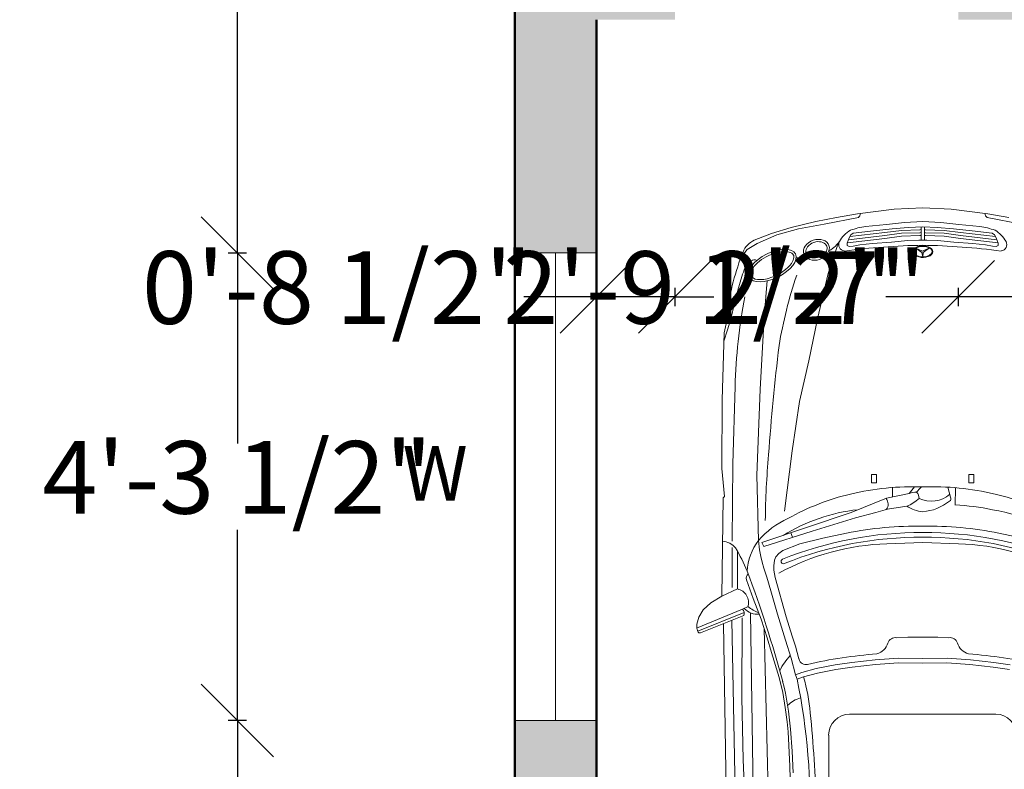
# Model space of a CAD drawing. Units: inches. Extents: x 3121 to 3511, y 1323 to 1998.
# Tile 3 of 10: x 3135 to 3244, y 1456 to 1539. Entities that reach past the tile are written whole.
import ezdxf

# ---------------------------------------------------------------- set-up
doc = ezdxf.new("R2010")
doc.units = ezdxf.units.IN
for name, color, linetype, lineweight in [('0_Equip', 250, 'Continuous', 13), ('A-ANNO-DIMS', 2, 'Continuous', 18), ('A-ANNO-TEXT', 7, 'Continuous', 18), ('A-GLAZ', 4, 'Continuous', 18), ('A-WALL', 7, 'Continuous', 50), ('A-WALL-PATT', 3, 'Continuous', 13)]:
    doc.layers.add(name, color=color, linetype=linetype, lineweight=lineweight)
doc.styles.get("Standard").update_dxf_attribs({"font": 'arial.ttf'})
doc.dimstyles.new('ISO-25', dxfattribs={"dimtxt": 8, "dimasz": 8, "dimexe": 1, "dimexo": 1, "dimtad": 0, "dimtih": 1, "dimtoh": 1, "dimlunit": 3, "dimtxsty": 'Standard', "dimblk": 'OBLIQUE', "dimcen": 2.5, "dimclrt": 1, "dimadec": 0, "dimazin": 0, "dimtfac": 1, "dimtmove": 0, "dimatfit": 3, "dimfxl": 1, "dimfxlon": 1, "dimarcsym": 0})

# ---------------------------------------------------------------- blocks, each defined once
blk = doc.blocks.new('A$C4C7B54D1')
at = {"layer": '0_Equip', "ltscale": 0.1}
for p, q in [((-1.0176, 2.6505), (-1.112, 2.6343)), ((-0.8531, 2.6707), (-1.0176, 2.6505)), ((-0.7257, 2.678), (-0.8531, 2.6707)), ((-0.7257, 2.678), (-0.5983, 2.6707)), ((-0.5983, 2.6707), (-0.4338, 2.6505)), ((-0.4338, 2.6505), (-0.3394, 2.6343)), ((-1.2037, 2.6168), (-1.3142, 2.5898)), ((-1.1673, 2.6045), (-1.2824, 2.5829)), ((-1.112, 2.6343), (-1.2037, 2.6168)), ((-1.0138, 2.6343), (-1.1673, 2.6045)), ((-0.8877, 2.6027), (-0.9812, 2.5937)), ((-0.8072, 2.6112), (-0.8877, 2.6027)), ((-0.7257, 2.6157), (-0.8072, 2.6112)), ((-0.7257, 2.6157), (-0.6441, 2.6112)), ((-0.6441, 2.6112), (-0.5636, 2.6027)), ((-0.5636, 2.6027), (-0.4701, 2.5937)), ((-0.4376, 2.6343), (-0.284, 2.6045)), ((-1.4032, 2.5628), (-1.4801, 2.5318)), ((-1.3142, 2.5898), (-1.4032, 2.5628)), ((-1.2824, 2.5829), (-1.3789, 2.557)), ((-1.4667, 2.5181), (-1.5113, 2.4907)), ((-1.3789, 2.557), (-1.4667, 2.5181)), ((-1.5113, 2.4907), (-1.5393, 2.4562)), ((-1.1083, 2.5037), (-1.1486, 2.3827)), ((-1.1486, 2.3827), (-1.1961, 2.1797)), ((-1.5353, 2.3701), (-1.5529, 2.308)), ((-1.435, 2.1869), (-1.4221, 2.3511)), ((-1.5529, 2.308), (-1.5677, 2.2486)), ((-1.5677, 2.2486), (-1.5849, 2.1795)), ((-1.6012, 2.2082), (-1.597, 2.1976)), ((-1.597, 2.1976), (-1.615, 2.1169)), ((-1.5849, 2.1795), (-1.5997, 2.1304)), ((-1.4537, 1.863), (-1.435, 2.1869)), ((-1.1961, 2.1797), (-1.2349, 1.9911)), ((-1.615, 2.1169), (-1.6235, 1.8165)), ((-1.5997, 2.1304), (-1.6161, 2.0798)), ((-1.2349, 1.9911), (-1.2767, 1.8097)), ((-1.566, 1.8774), (-1.5761, 1.5304)), ((-1.4681, 1.48), (-1.4537, 1.863)), ((-1.6235, 1.8165), (-1.6256, 1.5098)), ((-1.2767, 1.8097), (-1.3098, 1.588)), ((-1.3098, 1.588), (-1.3443, 1.3187)), ((-1.6256, 1.5098), (-1.6129, 1.3846)), ((-1.5761, 1.5304), (-1.5789, 1.1834)), ((-1.461, 1.1868), (-1.4681, 1.48)), ((-0.955, 1.4459), (-0.955, 1.4827)), ((-0.955, 1.4827), (-0.9321, 1.4827)), ((-0.9321, 1.4827), (-0.9321, 1.4459)), ((-0.5192, 1.4827), (-0.5192, 1.4459)), ((-0.4964, 1.4827), (-0.5192, 1.4827)), ((-0.4964, 1.4459), (-0.4964, 1.4827)), ((-0.9321, 1.4459), (-0.955, 1.4459)), ((-0.8614, 1.4242), (-0.8603, 1.382)), ((-0.6135, 1.4258), (-0.6012, 1.3814)), ((-0.5809, 1.3459), (-0.5793, 1.4233)), ((-0.5192, 1.4459), (-0.4964, 1.4459)), ((-1.6193, 1.3782), (-1.6252, 0.9375)), ((-1.6129, 1.3846), (-1.6193, 1.3782)), ((-0.8878, 1.3764), (-1.0456, 1.313)), ((-0.7861, 1.3973), (-0.8878, 1.3764)), ((-0.9361, 1.3119), (-0.8835, 1.3269)), ((-0.8835, 1.3269), (-0.7975, 1.3408)), ((-1.0456, 1.313), (-1.4462, 1.1776)), ((-1.2207, 1.2292), (-1.0263, 1.2883)), ((-1.0263, 1.2883), (-0.9361, 1.3119)), ((-1.4366, 1.1604), (-1.2207, 1.2292)), ((-1.3162, 1.2215), (-1.3088, 1.2011)), ((-1.1723, 1.1976), (-1.2762, 1.1716)), ((-1.0667, 1.22), (-1.1723, 1.1976)), ((-0.3847, 1.22), (-0.279, 1.1976)), ((-1.5793, 1.1562), (-1.5793, 0.9761)), ((-1.4565, 1.1447), (-1.461, 1.1868)), ((-1.4462, 1.1776), (-1.4366, 1.1604)), ((-1.2762, 1.1716), (-1.3515, 1.142)), ((-0.7257, 1.1776), (-0.8858, 1.1725)), ((-0.7257, 1.1776), (-0.5655, 1.1725)), ((-1.5552, 1.139), (-1.5552, 0.9693)), ((-1.4503, 1.1151), (-1.4565, 1.1447)), ((-1.444, 1.0892), (-1.4503, 1.1151)), ((-1.3828, 1.1133), (-1.39, 1.0981)), ((-1.3703, 1.1286), (-1.3828, 1.1133)), ((-1.3515, 1.142), (-1.3703, 1.1286)), ((-1.4368, 1.0623), (-1.444, 1.0892)), ((-1.4243, 1.0229), (-1.4368, 1.0623)), ((-1.39, 1.0981), (-1.3927, 1.0739)), ((-1.3927, 1.0739), (-1.3918, 1.0533)), ((-1.4064, 0.961), (-1.4243, 1.0229)), ((-1.3918, 1.0533), (-1.3867, 1.0211)), ((-1.3867, 1.0211), (-1.3374, 0.8446)), ((-1.5149, 1.011), (-1.4844, 0.9277)), ((-1.6252, 0.9375), (-1.6745, 0.908)), ((-1.6252, 0.9375), (-1.5546, 0.9696)), ((-1.4844, 0.9277), (-1.4486, 0.8345)), ((-1.3759, 0.8562), (-1.4064, 0.961)), ((-1.6745, 0.908), (-1.7088, 0.8764)), ((-1.508, 0.8914), (-1.5321, 0.8786)), ((-1.5321, 0.8786), (-1.7381, 0.7945)), ((-1.728, 0.8432), (-1.7366, 0.8127)), ((-1.5253, 0.865), (-1.7329, 0.7802)), ((-1.7088, 0.8764), (-1.728, 0.8432)), ((-1.5273, 0.8512), (-1.7203, 0.7738)), ((-1.5337, 0.8406), (-1.5355, 0.484)), ((-1.4835, -0.0735), (-1.497, 0.863)), ((-1.3401, 0.7406), (-1.3759, 0.8562)), ((-1.3374, 0.8446), (-1.3097, 0.7577)), ((-1.7366, 0.8127), (-1.7377, 0.7934)), ((-1.6171, 0.8152), (-1.5964, -0.6171)), ((-1.5805, 0.8299), (-1.5623, -0.138)), ((-1.4486, 0.8345), (-1.4226, 0.7503)), ((-1.7377, 0.7934), (-1.7327, 0.7794)), ((-1.4352, 0.792), (-1.4152, -0.045)), ((-1.4226, 0.7503), (-1.4029, 0.6849)), ((-1.3097, 0.7577), (-1.2953, 0.7129)), ((-0.7926, 0.7532), (-0.8418, 0.7514)), ((-0.7257, 0.7541), (-0.7926, 0.7532)), ((-0.7257, 0.7541), (-0.6587, 0.7532)), ((-0.6587, 0.7532), (-0.6095, 0.7514)), ((-1.315, 0.66), (-1.3401, 0.7406)), ((-1.2953, 0.7129), (-1.2801, 0.6573)), ((-1.4029, 0.6849), (-1.368, 0.5729)), ((-1.2951, 0.5849), (-1.315, 0.66)), ((-1.2801, 0.6573), (-1.2795, 0.6546)), ((-1.1177, 0.6302), (-1.2021, 0.6133)), ((-1.0437, 0.6403), (-1.1177, 0.6302)), ((-1.0411, 0.6196), (-1.1142, 0.6096)), ((-0.9389, 0.6526), (-1.0437, 0.6403)), ((-0.937, 0.6317), (-1.0411, 0.6196)), ((-0.8346, 0.6593), (-0.9389, 0.6526)), ((-0.834, 0.6384), (-0.937, 0.6317)), ((-0.7257, 0.6582), (-0.8346, 0.6593)), ((-0.7257, 0.6373), (-0.834, 0.6384)), ((-0.7257, 0.6582), (-0.6168, 0.6593)), ((-0.7257, 0.6373), (-0.6173, 0.6384)), ((-0.6173, 0.6384), (-0.5143, 0.6317)), ((-0.6168, 0.6593), (-0.5124, 0.6526)), ((-0.5143, 0.6317), (-0.4102, 0.6196)), ((-0.5124, 0.6526), (-0.4076, 0.6403)), ((-0.4102, 0.6196), (-0.3371, 0.6096)), ((-0.4076, 0.6403), (-0.3337, 0.6302)), ((-1.2663, 0.5956), (-1.2951, 0.5849)), ((-1.2879, 0.5653), (-1.2951, 0.5849)), ((-1.2599, 0.5757), (-1.2879, 0.5653)), ((-1.2021, 0.6133), (-1.2663, 0.5956)), ((-1.1973, 0.593), (-1.2599, 0.5757)), ((-1.1142, 0.6096), (-1.1973, 0.593)), ((-1.368, 0.5729), (-1.3527, 0.5066)), ((-1.3527, 0.5066), (-1.3411, 0.4394)), ((-1.5355, 0.484), (-1.5292, 0.2045)), ((-1.3411, 0.4394), (-1.3321, 0.3749)), ((-0.7257, 0.4085), (-1.0528, 0.4085)), ((-0.7257, 0.4085), (-0.3986, 0.4085)), ((-1.3321, 0.3749), (-1.3286, 0.3301)), ((-1.3286, 0.3301), (-1.3204, 0.1751)), ((-1.3178, 0.3418), (-1.31, 0.2426)), ((-1.1468, 0.3145), (-1.1468, 0.0145)), ((-1.31, 0.2426), (-1.306, 0.1454)), ((-1.5292, 0.2045), (-1.5185, -0.0974)), ((-1.3204, 0.1751), (-1.3164, 0.0193))]:
    blk.add_line(p, q, dxfattribs=at)
at = {"layer": '0_Equip'}
for p, q in [((-1.0475, 2.557), (-1.0545, 2.5425)), ((-1.0517, 2.5482), (-0.8949, 2.567)), ((-1.0364, 2.5634), (-1.0475, 2.557)), ((-0.9467, 2.5739), (-1.0364, 2.5634)), ((-0.8628, 2.5838), (-0.9467, 2.5739)), ((-0.8949, 2.567), (-0.8211, 2.5763)), ((-0.8949, 2.5537), (-0.8211, 2.5631)), ((-0.7905, 2.5897), (-0.8628, 2.5838)), ((-0.8211, 2.5763), (-0.738, 2.5791)), ((-0.8211, 2.5631), (-0.738, 2.5659)), ((-0.7257, 2.5926), (-0.7905, 2.5897)), ((-0.738, 2.5791), (-0.733, 2.58)), ((-0.738, 2.5659), (-0.733, 2.5668)), ((-0.733, 2.5923), (-0.733, 2.5325)), ((-0.7257, 2.5926), (-0.6608, 2.5897)), ((-0.7183, 2.5923), (-0.7183, 2.5325)), ((-0.7133, 2.5791), (-0.7183, 2.58)), ((-0.7133, 2.5659), (-0.7183, 2.5668)), ((-0.6302, 2.5763), (-0.7133, 2.5791)), ((-0.6302, 2.5631), (-0.7133, 2.5659)), ((-0.6608, 2.5897), (-0.5886, 2.5838)), ((-0.5564, 2.567), (-0.6302, 2.5763)), ((-0.5564, 2.5537), (-0.6302, 2.5631)), ((-0.5886, 2.5838), (-0.5046, 2.5739)), ((-0.3996, 2.5482), (-0.5564, 2.567)), ((-0.5046, 2.5739), (-0.4149, 2.5634)), ((-0.4149, 2.5634), (-0.4038, 2.557)), ((-0.4038, 2.557), (-0.3968, 2.5425)), ((-1.0545, 2.5425), (-1.0638, 2.5185)), ((-1.0638, 2.5185), (-1.0638, 2.5092)), ((-1.0631, 2.5204), (-0.8949, 2.5405)), ((-1.0577, 2.5343), (-0.8949, 2.5537)), ((-1.0067, 2.5116), (-0.9502, 2.5168)), ((-0.9502, 2.5168), (-0.8657, 2.5238)), ((-0.8949, 2.5405), (-0.8211, 2.5498)), ((-0.8657, 2.5238), (-0.7922, 2.5308)), ((-0.8211, 2.5498), (-0.738, 2.5526)), ((-0.7922, 2.5308), (-0.7433, 2.5325)), ((-0.7433, 2.5325), (-0.7257, 2.5325)), ((-0.738, 2.5526), (-0.733, 2.5536)), ((-0.708, 2.5325), (-0.7257, 2.5325)), ((-0.7133, 2.5526), (-0.7183, 2.5536)), ((-0.6302, 2.5498), (-0.7133, 2.5526)), ((-0.6591, 2.5308), (-0.708, 2.5325)), ((-0.5857, 2.5238), (-0.6591, 2.5308)), ((-0.5564, 2.5405), (-0.6302, 2.5498)), ((-0.5011, 2.5168), (-0.5857, 2.5238)), ((-0.3936, 2.5343), (-0.5564, 2.5537)), ((-0.3882, 2.5204), (-0.5564, 2.5405)), ((-0.4446, 2.5116), (-0.5011, 2.5168)), ((-0.3968, 2.5425), (-0.3875, 2.5185)), ((-0.3875, 2.5185), (-0.3875, 2.5092)), ((-1.0638, 2.5092), (-1.0545, 2.504)), ((-1.0545, 2.504), (-1.0376, 2.5051)), ((-1.0376, 2.5051), (-1.0067, 2.5116)), ((-0.7566, 2.4971), (-0.7261, 2.4828)), ((-0.7566, 2.4971), (-0.7291, 2.4776)), ((-0.7389, 2.5095), (-0.7395, 2.5059)), ((-0.7259, 2.4578), (-0.7291, 2.4776)), ((-0.6947, 2.4974), (-0.7261, 2.4828)), ((-0.7259, 2.4578), (-0.723, 2.4776)), ((-0.6947, 2.4974), (-0.723, 2.4776)), ((-0.7124, 2.5095), (-0.7119, 2.5059)), ((-0.4137, 2.5051), (-0.4446, 2.5116)), ((-0.3968, 2.504), (-0.4137, 2.5051)), ((-0.3875, 2.5092), (-0.3968, 2.504))]:
    blk.add_line(p, q, dxfattribs=at)
at = {"layer": '0_Equip', "ltscale": 0.1}
for centre, radius, start, end in [((-1.0252, 2.6508), 0.02, 304.7228, 3.5172), ((-0.4261, 2.6508), 0.02, 176.4828, 235.2772), ((-0.9799, 2.461), 0.1353, 120.8369, 151.2853), ((-0.9299, 2.2354), 0.3619, 98.1466, 109.2524), ((-0.5214, 2.2354), 0.3619, 70.7476, 81.8534), ((-0.4714, 2.461), 0.1353, 28.7147, 59.1631), ((-1.4391, 2.4422), 0.0986, 114.5945, 157.5113), ((-1.2153, 2.6098), 0.1432, 299.1564, 328.1831), ((-0.9799, 2.461), 0.1353, 151.2853, 161.5889), ((-1.0728, 2.5126), 0.029, 152.6038, 261.721), ((-0.3785, 2.5126), 0.029, 278.279, 27.3962), ((-0.4722, 2.0579), 1.139, 158.2564, 172.4203), ((-0.6679, -0.6671), 3.1773, 91.0415, 97.3969), ((-0.7834, -0.6671), 3.1773, 82.6031, 88.9585), ((-1.4083, 2.3394), 0.1306, 130.2084, 166.4224), ((-1.4798, 2.4259), 0.0184, 54.8052, 134.0204), ((-1.2841, 2.5028), 0.0501, 260.5448, 306.7068), ((0.5502, 1.746), 1.9445, 161.1117, 170.7019), ((1.1202, 1.7918), 2.6875, 169.5541, 178.1755), ((9.2655, 0.7813), 10.7109, 173.14258, 175.77374), ((2.9623, 1.2089), 4.3935, 175.2767, 179.1124), ((-0.7686, 0.201), 1.2267, 87.9955, 103.2364), ((-0.3726, 1.0935), 0.5131, 139.3585, 143.6922), ((-0.6528, 1.3354), 0.1211, 130.7679, 145.6911), ((-0.6828, 0.201), 1.2267, 76.7636, 92.0045), ((-0.786, 0.3109), 1.1158, 103.6551, 119.1148), ((-0.9216, 1.3498), 0.0409, 323.4512, 39.0343), ((-0.8494, 1.486), 0.1542, 289.6676, 314.192), ((-0.7554, 1.327), 0.0768, 88.1186, 113.6019), ((-0.7803, 1.3768), 0.0384, 357.9275, 44.3829), ((-0.6872, 1.4869), 0.1241, 243.8649, 311.6638), ((-0.6113, 1.3746), 0.0122, 294.8678, 33.6398), ((-0.6653, 0.3109), 1.1158, 60.8852, 76.3449), ((-0.929, 0.5266), 0.803, 96.22, 121.6991), ((-0.7147, 1.4628), 0.1474, 235.8143, 265.7174), ((-0.741, 1.5272), 0.212, 274.1513, 309.4931), ((-0.617, 0.3882), 0.9584, 77.6919, 87.8428), ((-0.5976, 0.2949), 1.0461, 55.3038, 79.8165), ((-1.1803, 0.9494), 0.3676, 113.8511, 139.7847), ((-0.7478, -0.378), 1.6295, 89.2231, 101.2856), ((-0.7036, -0.378), 1.6295, 78.7144, 90.7769), ((-0.7356, -0.4312), 1.6538, 89.6554, 111.9286), ((-0.7356, -0.4312), 1.6329, 89.6554, 111.9286), ((-0.7157, -0.4312), 1.6538, 68.0714, 90.3446), ((-0.7157, -0.4312), 1.6329, 68.0714, 90.3446), ((-1.6261, 1.102), 0.0813, 40.278, 87.0689), ((-2.3477, 0.6968), 0.9076, 22.824, 30.2904), ((-1.2706, 1.0395), 0.2408, 142.2718, 177.7746), ((-0.85, 0.0855), 1.0875, 91.8892, 118.6013), ((-0.6014, 0.0855), 1.0875, 61.3987, 88.1108), ((-1.3493, 1.0932), 0.0105, 111.9286, 291.9286), ((-1.4887, 1.0171), 0.0269, 132.3277, 193.1064), ((-6.6059, -0.8606), 5.4408, 15.0904, 20.5451), ((-1.5684, 0.9084), 0.0628, 344.3283, 77.2348), ((-1.463, 0.9441), 0.0879, 224.7932, 273.9292), ((-1.4233, 0.9849), 0.1262, 227.8287, 253.081), ((-1.5495, 0.8614), 0.0245, 335.4987, 44.5114), ((-1.7238, 0.7825), 0.00941, 199.646, 291.8616), ((-0.8474, 0.7163), 0.0355, 80.937, 162.15), ((-0.6039, 0.7163), 0.0355, 17.85, 99.063), ((-0.9515, 0.7495), 0.0737, 286.567, 342.4011), ((-0.4998, 0.7495), 0.0737, 197.5989, 253.433), ((-1.1535, 0.5061), 0.2334, 134.9877, 155.4049), ((-0.7896, -1.2957), 1.9795, 94.0807, 103.2045), ((-0.6617, -1.2957), 1.9795, 76.7955, 85.9193), ((-1.249, 0.662), 0.0314, 193.667, 283.2045), ((-2.0025, 0.3511), 0.7759, 4.7259, 16.8296), ((-2.6334, 0.2371), 1.3197, 4.5498, 13.9797), ((-4.2099, -0.0242), 2.9809, 358.1905, 11.4064), ((-1.2324, 0.3484), 0.1397, 106.6168, 134.6647), ((-6.5594, -0.126), 5.3575, 1.3159, 5.7952), ((-1.0528, 0.3145), 0.0941, 90, 180), ((-0.3986, 0.3145), 0.0941, 0, 90)]:
    blk.add_arc(centre, radius, start, end, dxfattribs=at)
for centre, major_axis, ratio in [((-1.2016, 2.4892), (0.0562, 0.0189), 0.759763), ((-1.399, 2.4187), (-0.1036, -0.0518), 0.497493)]:
    blk.add_ellipse(centre, major_axis=major_axis, ratio=ratio, dxfattribs=at)
at = {"layer": '0_Equip'}
blk.add_ellipse((-0.7253, 2.4812), major_axis=(-0.0426, 0), ratio=0.550187, dxfattribs=at)
at = {"layer": '0_Equip', "ltscale": 0.1}
for points, knots in [([(-1.1548, 2.5048), (-1.1596, 2.5191), (-1.1811, 2.5294), (-1.2283, 2.5198), (-1.248, 2.5001), (-1.2511, 2.4679), (-1.2373, 2.4539), (-1.1922, 2.4512), (-1.1656, 2.4658), (-1.1532, 2.4906), (-1.1526, 2.4983), (-1.1548, 2.5048)], [0, 0, 0, 0, 1.408119, 1.408119, 2.816238, 2.816238, 4.224358, 4.224358, 5.632477, 5.632477, 6.283185, 6.283185, 6.283185, 6.283185]), ([(-1.4937, 2.3714), (-1.4901, 2.3641), (-1.4809, 2.3581), (-1.4492, 2.3543), (-1.4277, 2.3571), (-1.3679, 2.3771), (-1.3298, 2.404), (-1.2994, 2.4483), (-1.2993, 2.4626), (-1.3171, 2.4801), (-1.3406, 2.4849), (-1.3989, 2.4733), (-1.4323, 2.4577), (-1.4816, 2.4186), (-1.4956, 2.3954), (-1.4959, 2.3774), (-1.4951, 2.3742), (-1.4937, 2.3714)], [0, 0, 0, 0, 0.646556, 0.646556, 1.293113, 1.293113, 2.410172, 2.410172, 3.309931, 3.309931, 4.20969, 4.20969, 5.109449, 5.109449, 6.031285, 6.031285, 6.283185, 6.283185, 6.283185, 6.283185])]:
    blk.add_open_spline(points, degree=3, knots=knots, dxfattribs=at)
at = {"layer": '0_Equip'}
blk.add_open_spline([(-0.7708, 2.4812), (-0.7708, 2.4725), (-0.7635, 2.4648), (-0.7294, 2.4499), (-0.6897, 2.4563), (-0.6733, 2.4916), (-0.7036, 2.5102), (-0.7526, 2.5051), (-0.7708, 2.4948), (-0.7708, 2.4812)], degree=3, knots=[0, 0, 0, 0, 0.903923, 0.903923, 2.878844, 2.878844, 4.872977, 4.872977, 6.283185, 6.283185, 6.283185, 6.283185], dxfattribs=at)
blk = doc.blocks.new('_Oblique')
at = {"color": 0, "linetype": 'ByBlock', "lineweight": -2}
blk.add_line((-0.5, -0.5), (0.5, 0.5), dxfattribs=at)
blk = doc.blocks.new('*D35')
at = {"layer": 'A-ANNO-DIMS', "color": 0, "lineweight": -2, "transparency": 16777216}
for p, q in [((3160.37, 1461.55), (3158.37, 1461.55)), ((3159.37, 1461.55), (3159.37, 1443.38)), ((3159.37, 1415.78), (3159.37, 1433.95)), ((3160.37, 1415.78), (3158.37, 1415.78))]:
    blk.add_line(p, q, dxfattribs=at)
at = {"layer": 'Defpoints', "color": 0, "transparency": 16777216}
for p in [(3159.37, 1461.55), (3189.92, 1461.55), (3189.92, 1415.78)]:
    blk.add_point(p, dxfattribs=at)
at = {"layer": 'A-ANNO-DIMS', "color": 0, "lineweight": -2, "transparency": 16777216, "xscale": 8, "yscale": 8, "zscale": 8}
for p, rotation in [((3159.37, 1461.55), 90), ((3159.37, 1415.78), 270)]:
    blk.add_blockref('_Oblique', p, dxfattribs=dict(at, rotation=rotation))
at = {"layer": 'A-ANNO-DIMS', "color": 1, "transparency": 16777216, "insert": (3159.37, 1438.67), "char_height": 8, "attachment_point": 5}
blk.add_mtext('3\'-10"', dxfattribs=at)
blk = doc.blocks.new('*D36')
at = {"layer": 'A-ANNO-DIMS', "color": 0, "lineweight": -2, "transparency": 16777216}
for p, q in [((3160.37, 1513.07), (3158.37, 1513.07)), ((3159.37, 1513.07), (3159.37, 1492.07)), ((3159.37, 1461.55), (3159.37, 1482.55)), ((3160.37, 1461.55), (3158.37, 1461.55))]:
    blk.add_line(p, q, dxfattribs=at)
at = {"layer": 'Defpoints', "color": 0, "transparency": 16777216}
for p in [(3159.37, 1513.07), (3189.92, 1513.07), (3189.92, 1461.55)]:
    blk.add_point(p, dxfattribs=at)
at = {"layer": 'A-ANNO-DIMS', "color": 0, "lineweight": -2, "transparency": 16777216, "xscale": 8, "yscale": 8, "zscale": 8}
for p, rotation in [((3159.37, 1513.07), 90), ((3159.37, 1461.55), 270)]:
    blk.add_blockref('_Oblique', p, dxfattribs=dict(at, rotation=rotation))
at = {"layer": 'A-ANNO-DIMS', "color": 1, "transparency": 16777216, "insert": (3159.37, 1487.31), "char_height": 8, "attachment_point": 5}
blk.add_mtext('4\'-3 1/2"', dxfattribs=at)
blk = doc.blocks.new('*D37')
at = {"layer": 'A-ANNO-DIMS', "color": 0, "lineweight": -2, "transparency": 16777216}
for p, q in [((3160.37, 1607.33), (3158.37, 1607.33)), ((3159.37, 1607.33), (3159.37, 1564.96)), ((3159.37, 1513.07), (3159.37, 1555.44)), ((3160.37, 1513.07), (3158.37, 1513.07))]:
    blk.add_line(p, q, dxfattribs=at)
at = {"layer": 'Defpoints', "color": 0, "transparency": 16777216}
for p in [(3159.37, 1607.33), (3189.92, 1607.33), (3189.92, 1513.07)]:
    blk.add_point(p, dxfattribs=at)
at = {"layer": 'A-ANNO-DIMS', "color": 0, "lineweight": -2, "transparency": 16777216, "xscale": 8, "yscale": 8, "zscale": 8}
for p, rotation in [((3159.37, 1607.33), 90), ((3159.37, 1513.07), 270)]:
    blk.add_blockref('_Oblique', p, dxfattribs=dict(at, rotation=rotation))
at = {"layer": 'A-ANNO-DIMS', "color": 1, "transparency": 16777216, "insert": (3159.37, 1560.2), "char_height": 8, "attachment_point": 5}
blk.add_mtext('7\'-10 1/2"', dxfattribs=at)
blk = doc.blocks.new('*D58')
at = {"layer": 'A-ANNO-DIMS', "color": 0, "lineweight": -2, "transparency": 16777216}
for p, q in [((3209.89, 1985.33), (3209.89, 1987.33)), ((3311.33, 1985.33), (3311.33, 1987.33)), ((3209.89, 1986.33), (3240.03, 1986.33)), ((3311.33, 1986.33), (3281.19, 1986.33))]:
    blk.add_line(p, q, dxfattribs=at)
at = {"layer": 'Defpoints', "color": 0, "transparency": 16777216}
for p in [(3311.33, 1986.33), (3209.89, 1424.78), (3311.33, 1424.78)]:
    blk.add_point(p, dxfattribs=at)
at = {"layer": 'A-ANNO-DIMS', "color": 0, "lineweight": -2, "transparency": 16777216, "xscale": 8, "yscale": 8, "zscale": 8, "rotation": 180}
blk.add_blockref('_Oblique', (3209.89, 1986.33), dxfattribs=at)
at = {"layer": 'A-ANNO-DIMS', "color": 0, "lineweight": -2, "transparency": 16777216, "xscale": 8, "yscale": 8, "zscale": 8}
blk.add_blockref('_Oblique', (3311.33, 1986.33), dxfattribs=at)
at = {"layer": 'A-ANNO-DIMS', "color": 1, "transparency": 16777216, "insert": (3260.61, 1986.33), "char_height": 8, "attachment_point": 5}
blk.add_mtext('8\'-5 1/2"', dxfattribs=at)
blk = doc.blocks.new('*D67')
at = {"layer": 'A-ANNO-DIMS', "color": 0, "lineweight": -2, "transparency": 16777216}
for p, q in [((3198.92, 1509.23), (3198.92, 1507.23)), ((3207.56, 1509.23), (3207.56, 1507.23)), ((3198.92, 1508.23), (3190.92, 1508.23)), ((3207.56, 1508.23), (3198.92, 1508.23))]:
    blk.add_line(p, q, dxfattribs=at)
at = {"layer": 'Defpoints', "color": 0, "transparency": 16777216}
for p in [(3198.92, 1538.78), (3207.56, 1538.78), (3198.92, 1508.23)]:
    blk.add_point(p, dxfattribs=at)
at = {"layer": 'A-ANNO-DIMS', "color": 0, "lineweight": -2, "transparency": 16777216, "xscale": 8, "yscale": 8, "zscale": 8, "rotation": 180}
blk.add_blockref('_Oblique', (3198.92, 1508.23), dxfattribs=at)
at = {"layer": 'A-ANNO-DIMS', "color": 0, "lineweight": -2, "transparency": 16777216, "xscale": 8, "yscale": 8, "zscale": 8}
blk.add_blockref('_Oblique', (3207.56, 1508.23), dxfattribs=at)
at = {"layer": 'A-ANNO-DIMS', "color": 1, "transparency": 16777216, "insert": (3170.34, 1508.23), "char_height": 8, "attachment_point": 5}
blk.add_mtext('0\'-8 1/2"', dxfattribs=at)
blk = doc.blocks.new('*D68')
at = {"layer": 'A-ANNO-DIMS', "color": 0, "lineweight": -2, "transparency": 16777216}
for p, q in [((3207.56, 1509.23), (3207.56, 1507.23)), ((3238.77, 1509.23), (3238.77, 1507.23)), ((3207.56, 1508.23), (3211.84, 1508.23)), ((3238.77, 1508.23), (3234.49, 1508.23))]:
    blk.add_line(p, q, dxfattribs=at)
at = {"layer": 'Defpoints', "color": 0, "transparency": 16777216}
for p in [(3207.56, 1538.78), (3238.77, 1538.78), (3207.56, 1508.23)]:
    blk.add_point(p, dxfattribs=at)
at = {"layer": 'A-ANNO-DIMS', "color": 0, "lineweight": -2, "transparency": 16777216, "xscale": 8, "yscale": 8, "zscale": 8, "rotation": 180}
blk.add_blockref('_Oblique', (3207.56, 1508.23), dxfattribs=at)
at = {"layer": 'A-ANNO-DIMS', "color": 0, "lineweight": -2, "transparency": 16777216, "xscale": 8, "yscale": 8, "zscale": 8}
blk.add_blockref('_Oblique', (3238.77, 1508.23), dxfattribs=at)
at = {"layer": 'A-ANNO-DIMS', "color": 1, "transparency": 16777216, "insert": (3223.16, 1508.23), "char_height": 8, "attachment_point": 5}
blk.add_mtext('2\'-7"', dxfattribs=at)
blk = doc.blocks.new('*D69')
at = {"layer": 'A-ANNO-DIMS', "color": 0, "lineweight": -2, "transparency": 16777216}
for p, q in [((3238.77, 1509.23), (3238.77, 1507.23)), ((3272.21, 1509.23), (3272.21, 1507.23)), ((3238.77, 1508.23), (3230.77, 1508.23)), ((3272.21, 1508.23), (3238.77, 1508.23))]:
    blk.add_line(p, q, dxfattribs=at)
at = {"layer": 'Defpoints', "color": 0, "transparency": 16777216}
for p in [(3238.77, 1538.78), (3272.21, 1538.78), (3238.77, 1508.23)]:
    blk.add_point(p, dxfattribs=at)
at = {"layer": 'A-ANNO-DIMS', "color": 0, "lineweight": -2, "transparency": 16777216, "xscale": 8, "yscale": 8, "zscale": 8, "rotation": 180}
blk.add_blockref('_Oblique', (3238.77, 1508.23), dxfattribs=at)
at = {"layer": 'A-ANNO-DIMS', "color": 0, "lineweight": -2, "transparency": 16777216, "xscale": 8, "yscale": 8, "zscale": 8}
blk.add_blockref('_Oblique', (3272.21, 1508.23), dxfattribs=at)
at = {"layer": 'A-ANNO-DIMS', "color": 1, "transparency": 16777216, "insert": (3210.12, 1508.23), "char_height": 8, "attachment_point": 5}
blk.add_mtext('2\'-9 1/2"', dxfattribs=at)

msp = doc.modelspace()

# ---------------------------------------------------------------- hatches: boundary and pattern name
at = {"layer": 'A-WALL-PATT'}
h = msp.add_hatch(color=256, dxfattribs=at)
h.dxf.hatch_style = 1
h.paths.add_polyline_path([(3274.023, 1955.784), (3189.918, 1955.784), (3189.918, 1910.219), (3198.918, 1910.219), (3198.918, 1946.784), (3259.023, 1946.784), (3259.023, 1921.61), (3261.023, 1921.61), (3261.023, 1946.784), (3274.023, 1946.784)])
h.paths.add_polyline_path([(3327.918, 1946.784), (3334.156, 1946.784), (3334.156, 1955.784), (3310.023, 1955.784), (3310.023, 1946.784), (3318.918, 1946.784), (3318.918, 1929.796), (3311.644, 1929.796), (3311.644, 1927.007), (3324.033, 1927.007), (3324.033, 1871.381), (3311.644, 1871.381), (3311.644, 1868.381), (3318.918, 1868.381), (3318.918, 1853.784), (3327.918, 1853.784)])
h.paths.add_polyline_path([(3456.918, 1955.784), (3384.562, 1955.784), (3384.562, 1946.784), (3447.918, 1946.784), (3447.918, 1877.779), (3456.918, 1877.779)])
h.paths.add_polyline_path([(3456.918, 1835.782), (3447.918, 1835.782), (3447.918, 1814.784), (3414.918, 1814.784), (3414.918, 1803.784), (3447.918, 1803.784), (3447.918, 1793.443), (3456.918, 1793.443)])
h.paths.add_polyline_path([(3456.918, 1558.434), (3447.918, 1558.434), (3447.918, 1547.784), (3375.918, 1547.784), (3375.918, 1598.784), (3378.918, 1598.784), (3378.918, 1602.284), (3375.918, 1602.284), (3375.918, 1674.284), (3369.918, 1674.284), (3369.918, 1547.784), (3364.418, 1547.784), (3364.418, 1538.784), (3447.918, 1538.784), (3447.918, 1512.628), (3456.918, 1512.628)])
h.paths.add_polyline_path([(3456.918, 1460.558), (3447.918, 1460.558), (3447.918, 1424.784), (3412.543, 1424.784), (3412.543, 1415.784), (3456.918, 1415.784)])
h.paths.add_polyline_path([(3358.149, 1424.784), (3322.918, 1424.784), (3322.918, 1538.784), (3328.418, 1538.784), (3328.418, 1547.784), (3308.208, 1547.784), (3308.208, 1538.784), (3318.918, 1538.784), (3318.918, 1424.784), (3311.328, 1424.784), (3311.328, 1415.784), (3358.149, 1415.784)])
h.paths.add_polyline_path([(3207.562, 1547.784), (3198.918, 1547.784), (3198.918, 1607.327), (3189.918, 1607.327), (3189.918, 1513.073), (3198.918, 1513.073), (3198.918, 1538.784), (3207.562, 1538.784)])
h.paths.add_polyline_path([(3198.918, 1461.548), (3189.918, 1461.548), (3189.918, 1415.784), (3209.892, 1415.784), (3209.892, 1424.784), (3198.918, 1424.784)])
h.paths.add_polyline_path([(3272.208, 1547.784), (3238.766, 1547.784), (3238.766, 1538.784), (3272.208, 1538.784)])
h.paths.add_polyline_path([(3261.023, 1748.784), (3198.918, 1748.784), (3198.918, 1768.387), (3189.918, 1768.387), (3189.918, 1692.279), (3198.918, 1692.279), (3198.918, 1739.784), (3261.023, 1739.784)])
h.paths.add_polyline_path([(3198.918, 1856.171), (3189.918, 1856.171), (3189.918, 1808.331), (3198.918, 1808.331), (3198.918, 1821.074), (3261.023, 1821.074), (3261.023, 1862.309), (3259.023, 1862.309), (3259.023, 1825.074), (3198.918, 1825.074)])

# ---------------------------------------------------------------- linework, layer by layer
at = {"layer": 'A-GLAZ'}
for p, q in [((3198.918, 1513.073), (3189.918, 1513.073)), ((3194.418, 1461.548), (3194.418, 1513.073)), ((3198.918, 1461.548), (3189.918, 1461.548))]:
    msp.add_line(p, q, dxfattribs=at)
at = {"layer": 'A-WALL'}
for p, q in [((3189.918, 1955.784), (3189.918, 1415.784)), ((3198.918, 1538.784), (3198.918, 1424.784))]:
    msp.add_line(p, q, dxfattribs=at)

# ---------------------------------------------------------------- block references
at = {"layer": '0_Equip', "xscale": 24.59625072819005, "yscale": 24.59625072819005, "zscale": 24.59625072819005}
msp.add_blockref('A$C4C7B54D1', (3252.699, 1452.199), dxfattribs=at)

# ---------------------------------------------------------------- texts
at = {"layer": 'A-ANNO-TEXT', "insert": (3174.942, 1491.797), "char_height": 6, "attachment_point": 1}
msp.add_mtext_dynamic_manual_height_columns('\\pxqc;W', width=12.42925, gutter_width=12.5, heights=[0], dxfattribs=at)

# ---------------------------------------------------------------- dimensions: what is measured, and where the dimension line sits
at = {"layer": 'A-ANNO-DIMS'}
dim = msp.add_linear_dim(base=(3311.328, 1986.334), p1=(3209.892, 1424.784), p2=(3311.328, 1424.784), dimstyle='ISO-25', override={"dimdec": 1, "dimlfac": 1, "dimrnd": 0, "dimzin": 1, "dimdsep": 46, "dimlunit": 4, "dimfrac": 2}, dxfattribs=at)
dim.commit()
dim.dimension.update_dxf_attribs({"geometry": '*D58', "text_midpoint": (3260.61, 1986.334)})
for base, p1, p2, angle, picture, middle in [((3159.368, 1607.327), (3189.918, 1513.073), (3189.918, 1607.327), 90, '*D37', (3159.368, 1560.2)), ((3198.918, 1508.234), (3207.562, 1538.784), (3198.918, 1538.784), 180, '*D67', (3170.339, 1508.234)), ((3238.766, 1508.234), (3272.208, 1538.784), (3238.766, 1538.784), 180, '*D69', (3210.119, 1508.234)), ((3207.562, 1508.234), (3238.766, 1538.784), (3207.562, 1538.784), 180, '*D68', (3223.164, 1508.234)), ((3159.368, 1513.073), (3189.918, 1461.548), (3189.918, 1513.073), 90, '*D36', (3159.368, 1487.311)), ((3159.368, 1461.548), (3189.918, 1415.784), (3189.918, 1461.548), 90, '*D35', (3159.368, 1438.666))]:
    dim = msp.add_linear_dim(base=base, p1=p1, p2=p2, angle=angle, dimstyle='ISO-25', override={"dimdec": 1, "dimlfac": 1, "dimrnd": 0, "dimzin": 1, "dimdsep": 46, "dimlunit": 4, "dimfrac": 2}, dxfattribs=at)
    dim.commit()
    dim.dimension.update_dxf_attribs({"geometry": picture, "text_midpoint": middle})

doc.saveas('drawing.dxf')
